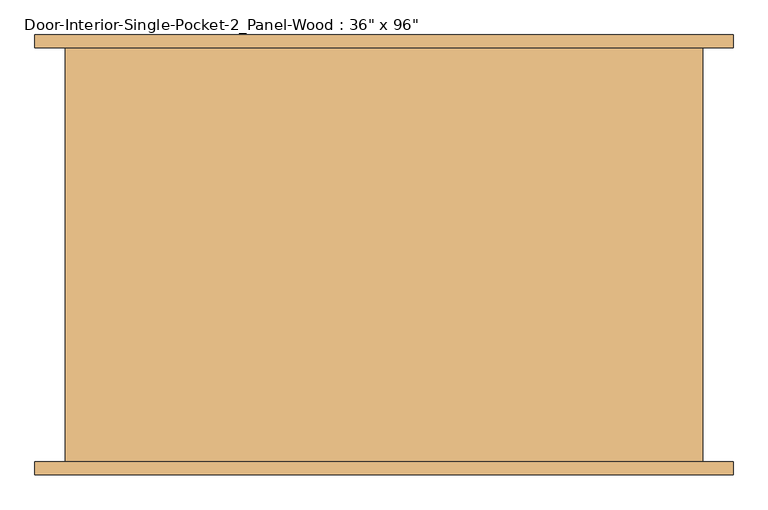
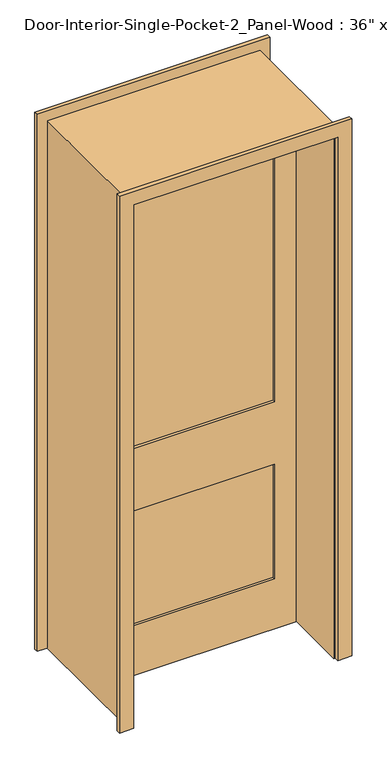
"""IFC4 building model written with IfcOpenShell, lengths in millimetres: door geometry."""

from ifc_helpers import new_model, si_unit, frame, origin, place, context, project, spatial, polyline, outline, extrude, faceted_brep, source, transform, mapped, element, save


def door_ede55593(model_context):
    return source(origin(), model_context, "Body", "SolidModel", [
        extrude(outline(polyline([(0.0, 438.15), (0.0, 501.65), (2508.25, 501.65), (2508.25, -527.05), (0.0, -527.05), (0.0, -463.55), (2444.75, -463.55), (2444.75, 438.15), (0.0, 438.15)])), frame((0.0, -323.85, 0.0), z_axis=(0.0, 1.0, 0.0), x_axis=(0.0, 0.0, 1.0)), (0.0, 0.0, 1.0), 19.05),
        extrude(outline(polyline([(0.0, 438.15), (0.0, 501.65), (2508.25, 501.65), (2508.25, -527.05), (0.0, -527.05), (0.0, -463.55), (2444.75, -463.55), (2444.75, 438.15), (0.0, 438.15)])), frame((0.0, 304.8, 0.0), z_axis=(0.0, 1.0, 0.0), x_axis=(0.0, 0.0, 1.0)), (0.0, 0.0, 1.0), 19.05),
        faceted_brep([(457.2, -304.8, 0.0), (457.2, -17.4625, 0.0), (457.2, -17.4625, 2438.4), (457.2, 17.4625, 2438.4), (457.2, 17.4625, 0.0), (457.2, 304.8, 0.0), (457.2, 304.8, 2463.8), (457.2, -304.8, 2463.8), (-482.6, -304.8, 2463.8), (-482.6, -304.8, 0.0), (-457.2, -304.8, 0.0), (-457.2, -304.8, 2438.4), (431.8, -304.8, 2438.4), (431.8, -304.8, 0.0), (-457.2, 304.8, 2438.4), (431.8, 304.8, 2438.4), (431.8, 17.4625, 2438.4), (431.8, -17.4625, 2438.4), (431.8, 304.8, 0.0), (-457.2, 304.8, 0.0), (-482.6, 304.8, 0.0), (-482.6, 304.8, 2463.8), (431.8, -17.4625, 0.0), (431.8, 17.4625, 0.0)], [[[0, 1, 2, 3, 4, 5, 6, 7]], [[0, 7, 8, 9, 10, 11, 12, 13]], [[11, 14, 15, 16, 3, 2, 17, 12]], [[6, 5, 18, 15, 14, 19, 20, 21]], [[6, 21, 8, 7]], [[10, 9, 20, 19]], [[11, 10, 19, 14]], [[9, 8, 21, 20]], [[1, 0, 13, 22]], [[5, 4, 23, 18]], [[18, 23, 16, 15]], [[23, 4, 3, 16]], [[1, 22, 17, 2]], [[22, 13, 12, 17]]]),
        extrude(outline(polyline([(336.55, -5.8208333), (-336.55, -5.8208333), (-336.55, 5.8208333), (336.55, 5.8208333), (336.55, -5.8208333)])), frame((0.0, 0.0, 1060.45), z_axis=(0.0, 0.0, 1.0), x_axis=(1.0, 0.0, 0.0)), (0.0, 0.0, 1.0), 1258.8875),
        extrude(outline(polyline([(336.55, -5.8208333), (-336.55, -5.8208333), (-336.55, 5.8208333), (336.55, 5.8208333), (336.55, -5.8208333)])), frame((0.0, 0.0, 231.775), z_axis=(0.0, 0.0, 1.0), x_axis=(1.0, 0.0, 0.0)), (0.0, 0.0, 1.0), 536.575),
        extrude(outline(polyline([(2438.4, -457.2), (0.0, -457.2), (0.0, 457.2), (2438.4, 457.2), (2438.4, -457.2)]), holes=[polyline([(2319.3375, -336.55), (2319.3375, 336.55), (1060.45, 336.55), (1060.45, -336.55), (2319.3375, -336.55)]), polyline([(768.35, -336.55), (768.35, 336.55), (231.775, 336.55), (231.775, -336.55), (768.35, -336.55)])]), frame((0.0, -17.4625, 0.0), z_axis=(0.0, 1.0, 0.0), x_axis=(0.0, 0.0, 1.0)), (0.0, 0.0, 1.0), 34.925),
    ])


if __name__ == "__main__":
    model = new_model("IFC4")
    model_context = context("Model", 3, world=origin())
    ifc_project = project(units=[si_unit("LENGTHUNIT", "METRE", prefix="MILLI")], contexts=[model_context])
    site = spatial("IfcSite", under=ifc_project)
    building = spatial("IfcBuilding", under=site)
    placement = place(None, origin())
    door_shape = door_ede55593(model_context)
    element("IfcDoor", 1, ObjectType="Door-Interior-Single-Pocket-2_Panel-Wood : 36\" x 96\"", at=placement, inside=building, context=model_context, shape_type="MappedRepresentation", body=[
        mapped(door_shape, transform((0.0, 0.0, 0.0), x_axis=(1.0, 0.0, 0.0), y_axis=(0.0, 1.0, 0.0), z_axis=(0.0, 0.0, 1.0))),
    ])
    save(model, "model.ifc")

# Revit data of these elements
# Type "Door-Interior-Single-Pocket-2_Panel-Wood : 36\" x 96\""
#   Type Mark = "8"
#   Assembly Code = "C1020300"
#   Analytic Construction = "Wooden"
#   Top Rail = 0' - 4 11/16"
#   Thickness = 0' - 1 3/8"
#   Thermal Resistance (R) = 0.455703 (m²·K)/W
#   Stiles = 0' - 4 3/4"
#   Rough Width = 6' - 1"
#   Rough Height = 8' - 4 1/2"
#   Lock Rail = 0' - 7 1/2"
#   Location [instance default] = 3' - 0"
#   Height = 8' - 0"
#   Width = 3' - 0"
#   Heat Transfer Coefficient (U) = 2.19465 W/(m²·K)
#   Bottom Rail = 0' - 9 1/8"
#   Panel Open [instance default] = no
#   Trim Material = Cherry
#   Panel Material = Cherry
#   Frame Material = Cherry
#   Visual Light Transmittance = 0
#   Solar Heat Gain Coefficient = 0
#   Wall Closure = (empty or 0)
#   Function = (empty or 0)
# Element 1 (IfcDoor, "Door-Interior-Single-Pocket-2_Panel-Wood : 36\" x 96\"")
#   Materials on its faces: "Cherry"
# Materials
#   "Cherry": class "Wood", colour RGB 226 177 128, transparency 0, Description = "Prunus Serotina", Cost = 0
